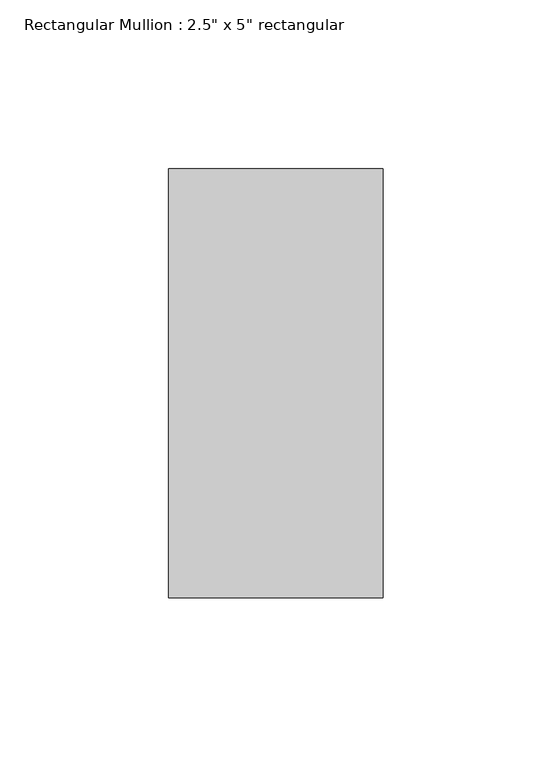
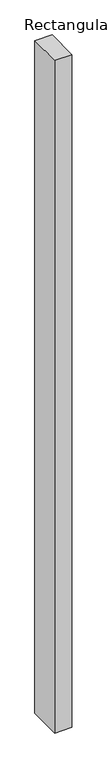
"""IFC4 building model written with IfcOpenShell, lengths in millimetres: member geometry."""

from ifc_helpers import new_model, si_unit, frame, origin, place, context, project, spatial, polyline, outline, extrude, source, transform, mapped, element, save


def member_1631f5ff(model_context):
    return source(origin(), model_context, "Body", "SweptSolid", [
        extrude(outline(polyline([(31.75, 63.5), (31.75, -63.5), (-31.75, -63.5), (-31.75, 63.5), (31.75, 63.5)])), frame((0.0, 0.0, -2641.6), z_axis=(0.0, 0.0, 1.0), x_axis=(1.0, 0.0, 0.0)), (0.0, 0.0, 1.0), 2641.6),
    ])


if __name__ == "__main__":
    model = new_model("IFC4")
    model_context = context("Model", 3, world=origin())
    ifc_project = project(units=[si_unit("LENGTHUNIT", "METRE", prefix="MILLI")], contexts=[model_context])
    site = spatial("IfcSite", under=ifc_project)
    building = spatial("IfcBuilding", under=site)
    placement = place(None, origin())
    member_shape = member_1631f5ff(model_context)
    element("IfcMember", 1, ObjectType="Rectangular Mullion : 2.5\" x 5\" rectangular", at=placement, inside=building, context=model_context, shape_type="MappedRepresentation", body=[
        mapped(member_shape, transform((0.0, 0.0, 0.0), x_axis=(1.0, 0.0, 0.0), y_axis=(0.0, 1.0, 0.0), z_axis=(0.0, 0.0, 1.0))),
    ])
    save(model, "model.ifc")

# Revit data of these elements
# Type "Rectangular Mullion : 2.5\" x 5\" rectangular"
#   built-in parameter 1007304 = 0.416667 (stored number, unit not read)
#   built-in parameter 1007301 = 0.104167 (stored number, unit not read)
#   built-in parameter 1007300 = 0.104167 (stored number, unit not read)
# Element 1 (IfcMember, "Rectangular Mullion : 2.5\" x 5\" rectangular")
#   Materials on its faces: "Aluminum"
# Materials
#   "Aluminum": class "Metal", colour RGB 247 247 247, transparency 0, Description = "Aluminum 6061", Cost = 0
